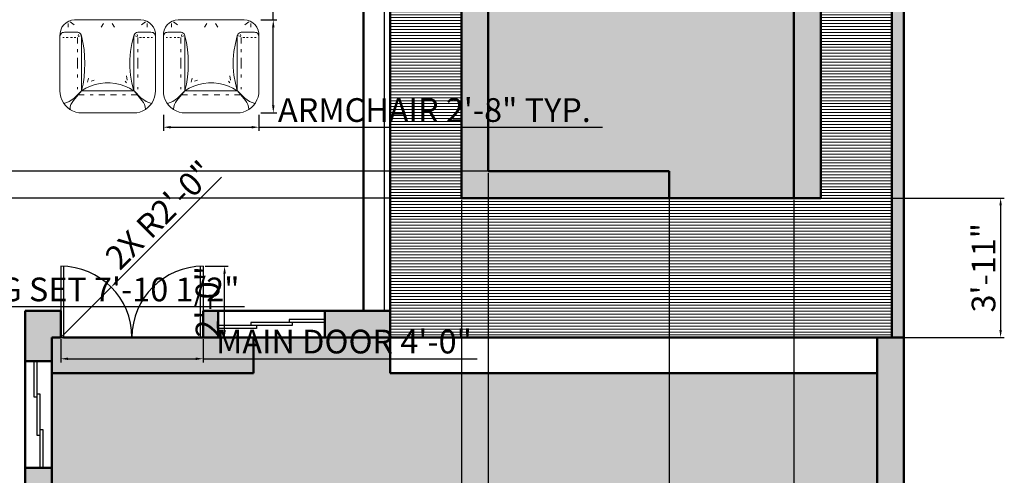
# Model space of a CAD drawing. Units: inches. Extents: x 1770 to 3141, y 984 to 1614.
# Tile 6 of 12: x 2115 to 2447, y 1254 to 1407. Entities that reach past the tile are written whole.
import ezdxf

# ---------------------------------------------------------------- set-up
doc = ezdxf.new("R2010")
doc.units = ezdxf.units.IN
for name, color, linetype, lineweight in [('A-ANNO-DIMS', 2, 'Continuous', 18), ('A-DOOR', 4, 'Continuous', 25), ('A-FLOR-PATT', 252, 'Continuous', 13), ('A-FURN', 8, 'Continuous', 18), ('A-GLAZ', 5, 'Continuous', 25), ('A-WALL', 7, 'Continuous', 50), ('A-WALL-PATT', 8, 'Continuous', 13)]:
    doc.layers.add(name, color=color, linetype=linetype, lineweight=lineweight)
doc.styles.get("Standard").update_dxf_attribs({"font": 'arial.ttf'})
doc.dimstyles.new('ISO-25', dxfattribs={"dimtxt": 8, "dimasz": 2.5, "dimexe": 1.25, "dimexo": 0.625, "dimtad": 1, "dimdec": 1, "dimlunit": 3, "dimtxsty": 'Standard', "dimcen": 2.5, "dimclrt": 1, "dimadec": 0, "dimazin": 0, "dimtfac": 1, "dimtdec": 1, "dimtmove": 0, "dimatfit": 3, "dimfxl": 1, "dimarcsym": 0})

# ---------------------------------------------------------------- blocks, each defined once
blk = doc.blocks.new("MD D 4'")
for p, q in [((0, 24), (0, 0)), ((1, 24), (1, 0)), ((47, 24), (47, 0)), ((48, 24), (48, 0)), ((0, 0), (1, 0)), ((48, 0), (47, 0))]:
    blk.add_line(p, q)
for centre, start, end in [((0, 0), 0, 90), ((48, 0), 90, 180)]:
    blk.add_arc(centre, 24, start, end)
blk = doc.blocks.new('sofa-47')
at = {"color": 0, "linetype": 'ByBlock'}
for p, q in [((-0.1449, 0.828), (-0.1656, 0.81)), ((-0.1449, 0.828), (-0.1656, 0.81)), ((-0.1206, 0.8424), (-0.1449, 0.828)), ((-0.1206, 0.8424), (-0.1449, 0.828)), ((-0.126, 0.8208), (-0.126, 0.7884)), ((-0.0945, 0.8514), (-0.1206, 0.8424)), ((-0.0945, 0.8514), (-0.1206, 0.8424)), ((-0.072, 0.8109), (-0.108, 0.8379)), ((-0.0666, 0.855), (-0.0945, 0.8514)), ((-0.0666, 0.855), (-0.0945, 0.8514)), ((0.2376, 0.855), (-0.0666, 0.855)), ((0.2376, 0.855), (-0.0666, 0.855)), ((0.1764, 0.7884), (0.198, 0.8235)), ((0.5418, 0.855), (0.2376, 0.855)), ((0.5418, 0.855), (0.2376, 0.855)), ((0.2772, 0.8235), (0.2988, 0.7884)), ((0.5697, 0.8514), (0.5418, 0.855)), ((0.5697, 0.8514), (0.5418, 0.855)), ((0.5472, 0.8109), (0.5832, 0.8379)), ((0.5958, 0.8424), (0.5697, 0.8514)), ((0.5958, 0.8424), (0.5697, 0.8514)), ((0.6201, 0.828), (0.5958, 0.8424)), ((0.6201, 0.828), (0.5958, 0.8424)), ((0.6012, 0.8208), (0.6012, 0.7884)), ((0.6408, 0.81), (0.6201, 0.828)), ((0.6408, 0.81), (0.6201, 0.828)), ((-0.2007, 0.7344), (-0.2016, 0.7065)), ((-0.2007, 0.7344), (-0.2016, 0.7065)), ((-0.1944, 0.7614), (-0.2007, 0.7344)), ((-0.1944, 0.7614), (-0.2007, 0.7344)), ((-0.1989, 0.7164), (-0.1944, 0.7254)), ((-0.1827, 0.7875), (-0.1944, 0.7614)), ((-0.1827, 0.7875), (-0.1944, 0.7614)), ((-0.1944, 0.7254), (-0.1872, 0.7326)), ((-0.1872, 0.7326), (-0.1791, 0.738)), ((-0.1656, 0.81), (-0.1827, 0.7875)), ((-0.1656, 0.81), (-0.1827, 0.7875)), ((-0.1791, 0.738), (-0.1692, 0.7407)), ((-0.1692, 0.7407), (-0.1593, 0.7416)), ((-0.1593, 0.7416), (-0.0486, 0.7416)), ((-0.0486, 0.7416), (-0.0378, 0.7416)), ((-0.0378, 0.7416), (-0.0279, 0.7389)), ((-0.0279, 0.7389), (-0.0189, 0.7335)), ((-0.0189, 0.7335), (-0.0117, 0.7263)), ((-0.0117, 0.7263), (-0.0063, 0.7182)), ((0.4815, 0.7182), (0.4869, 0.7263)), ((0.4869, 0.7263), (0.4941, 0.7335)), ((0.4941, 0.7335), (0.5031, 0.7389)), ((0.5031, 0.7389), (0.513, 0.7416)), ((0.513, 0.7416), (0.5238, 0.7416)), ((0.5238, 0.7416), (0.6345, 0.7416)), ((0.6345, 0.7416), (0.6444, 0.7407)), ((0.6579, 0.7875), (0.6408, 0.81)), ((0.6579, 0.7875), (0.6408, 0.81)), ((0.6444, 0.7407), (0.6543, 0.738)), ((0.6543, 0.738), (0.6624, 0.7326)), ((0.6696, 0.7614), (0.6579, 0.7875)), ((0.6696, 0.7614), (0.6579, 0.7875)), ((0.6624, 0.7326), (0.6696, 0.7254)), ((0.6759, 0.7344), (0.6696, 0.7614)), ((0.6759, 0.7344), (0.6696, 0.7614)), ((0.6696, 0.7254), (0.6741, 0.7164)), ((0.6768, 0.7065), (0.6759, 0.7344)), ((0.6768, 0.7065), (0.6759, 0.7344)), ((-0.2016, 0.7065), (-0.1989, 0.7164)), ((-0.2016, 0.7065), (-0.2016, 0.2034)), ((-0.2016, 0.2034), (-0.2016, 0.7065)), ((-0.1746, 0.693), (-0.162, 0.693)), ((-0.1431, 0.693), (-0.126, 0.693)), ((-0.1035, 0.693), (-0.0864, 0.693)), ((-0.072, 0.693), (-0.054, 0.693)), ((-0.0396, 0.693), (-0.0396, 0.639)), ((-0.0351, 0.7074), (-0.0324, 0.72)), ((-0.0351, 0.7029), (-0.0126, 0.7074)), ((-0.0063, 0.7182), (-0.0027, 0.7083)), ((0.0099, 0.6462), (-0.0027, 0.7083)), ((-0.0027, 0.7083), (-0.0027, 0.6975)), ((-0.0027, 0.6975), (-0.0027, 0.2034)), ((0.0198, 0.5832), (0.0099, 0.6462)), ((0.4599, 0.6372), (0.4473, 0.5652)), ((0.4779, 0.7083), (0.4599, 0.6372)), ((0.4779, 0.7083), (0.4815, 0.7182)), ((0.4779, 0.6975), (0.4779, 0.7083)), ((0.4779, 0.2034), (0.4779, 0.6975)), ((0.5103, 0.7029), (0.4878, 0.7074)), ((0.5103, 0.7074), (0.5076, 0.72)), ((0.5148, 0.693), (0.5148, 0.639)), ((0.5472, 0.693), (0.5292, 0.693)), ((0.5787, 0.693), (0.5616, 0.693)), ((0.6183, 0.693), (0.6012, 0.693)), ((0.6498, 0.693), (0.6372, 0.693)), ((0.6741, 0.7164), (0.6768, 0.7065)), ((0.6768, 0.2034), (0.6768, 0.7065)), ((0.6768, 0.7065), (0.6768, 0.2034)), ((-0.0396, 0.585), (-0.0396, 0.558)), ((0.0252, 0.5193), (0.0198, 0.5832)), ((0.4473, 0.5652), (0.441, 0.4923)), ((0.5148, 0.585), (0.5148, 0.558)), ((-0.0396, 0.4077), (-0.0396, 0.5067)), ((0.027, 0.4554), (0.0252, 0.5193)), ((0.0252, 0.3924), (0.027, 0.4554)), ((0.441, 0.4923), (0.441, 0.4194)), ((0.5148, 0.4077), (0.5148, 0.5067)), ((0.0198, 0.3285), (0.0252, 0.3924)), ((0.441, 0.4194), (0.4473, 0.3465)), ((-0.0396, 0.3267), (-0.0396, 0.3537)), ((0.0108, 0.2655), (0.0198, 0.3285)), ((0.0531, 0.2826), (0.0621, 0.3186)), ((0.0855, 0.2907), (0.1116, 0.3015)), ((0.1683, 0.2718), (0.1233, 0.2619)), ((0.2142, 0.2763), (0.1683, 0.2718)), ((0.261, 0.2763), (0.2142, 0.2763)), ((0.3069, 0.2718), (0.261, 0.2763)), ((0.3519, 0.2619), (0.3069, 0.2718)), ((0.4104, 0.2781), (0.3969, 0.2934)), ((0.4167, 0.3015), (0.4104, 0.3402)), ((0.4473, 0.3465), (0.4599, 0.2745)), ((0.4599, 0.2745), (0.4779, 0.2034)), ((0.5148, 0.3267), (0.5148, 0.3537)), ((-0.2016, 0.2034), (-0.1998, 0.1746)), ((-0.1998, 0.1746), (-0.2016, 0.2034)), ((-0.0765, 0.1152), (-0.0045, 0.2016)), ((-0.0045, 0.2016), (-0.0711, 0.135)), ((-0.0396, 0.2187), (-0.0396, 0.2358)), ((-0.0027, 0.2034), (0.0108, 0.2655)), ((0.0369, 0.2277), (-0.0027, 0.2034)), ((-0.0027, 0.2034), (0.2376, 0.2034)), ((0.0792, 0.2466), (0.0369, 0.2277)), ((0.1233, 0.2619), (0.0792, 0.2466)), ((0.2376, 0.2034), (0.4779, 0.2034)), ((0.396, 0.2466), (0.3519, 0.2619)), ((0.4383, 0.2277), (0.396, 0.2466)), ((0.4779, 0.2034), (0.4383, 0.2277)), ((0.4797, 0.2016), (0.5517, 0.1152)), ((0.5463, 0.135), (0.4797, 0.2016)), ((0.5148, 0.2187), (0.5148, 0.2358)), ((0.675, 0.1746), (0.6768, 0.2034)), ((0.6768, 0.2034), (0.675, 0.1746)), ((-0.1998, 0.1746), (-0.1935, 0.1458)), ((-0.1935, 0.1458), (-0.1998, 0.1746)), ((-0.1935, 0.1458), (-0.1836, 0.1188)), ((-0.1836, 0.1188), (-0.1935, 0.1458)), ((-0.1836, 0.1188), (-0.1701, 0.0936)), ((-0.1701, 0.0936), (-0.1836, 0.1188)), ((-0.1701, 0.0936), (-0.153, 0.0702)), ((-0.153, 0.0702), (-0.1701, 0.0936)), ((-0.1395, 0.0954), (-0.1647, 0.0873)), ((-0.1152, 0.1062), (-0.1395, 0.0954)), ((-0.0927, 0.1197), (-0.1152, 0.1062)), ((-0.0999, 0.0774), (-0.09, 0.0972)), ((-0.0711, 0.135), (-0.0927, 0.1197)), ((-0.09, 0.0972), (-0.0765, 0.1152)), ((-0.0324, 0.1647), (0.0216, 0.1647)), ((0.0756, 0.1647), (0.1026, 0.1647)), ((0.1566, 0.1647), (0.2106, 0.1647)), ((0.3186, 0.1647), (0.2646, 0.1647)), ((0.3996, 0.1647), (0.3726, 0.1647)), ((0.5076, 0.1647), (0.4536, 0.1647)), ((0.5679, 0.1197), (0.5463, 0.135)), ((0.5517, 0.1152), (0.5652, 0.0972)), ((0.5652, 0.0972), (0.5751, 0.0774)), ((0.5904, 0.1062), (0.5679, 0.1197)), ((0.6147, 0.0954), (0.5904, 0.1062)), ((0.6399, 0.0873), (0.6147, 0.0954)), ((0.6282, 0.0702), (0.6453, 0.0936)), ((0.6453, 0.0936), (0.6282, 0.0702)), ((0.6453, 0.0936), (0.6588, 0.1188)), ((0.6588, 0.1188), (0.6453, 0.0936)), ((0.6588, 0.1188), (0.6687, 0.1458)), ((0.6687, 0.1458), (0.6588, 0.1188)), ((0.6687, 0.1458), (0.675, 0.1746)), ((0.675, 0.1746), (0.6687, 0.1458)), ((-0.153, 0.0702), (-0.1323, 0.0495)), ((-0.1323, 0.0495), (-0.153, 0.0702)), ((-0.1323, 0.0495), (-0.1082, 0.0312)), ((-0.1098, 0.0324), (-0.1323, 0.0495)), ((-0.0846, 0.018), (-0.1098, 0.0324)), ((-0.1082, 0.0312), (-0.1081, 0.0315)), ((-0.1081, 0.0315), (-0.0846, 0.018)), ((-0.108, 0.0333), (-0.1062, 0.0558)), ((-0.1062, 0.0558), (-0.0999, 0.0774)), ((-0.0846, 0.018), (-0.0567, 0.0081)), ((-0.0567, 0.0081), (-0.0846, 0.018)), ((-0.0567, 0.0081), (-0.0288, 0.0018)), ((-0.0288, 0.0018), (-0.0567, 0.0081)), ((-0.0288, 0.0018), (0, 0)), ((0, 0), (-0.0288, 0.0018)), ((0, 0), (0.2376, 0)), ((0.2376, 0), (0, 0)), ((0.2376, 0), (0.4752, 0)), ((0.4752, 0), (0.2376, 0)), ((0.4752, 0), (0.504, 0.0018)), ((0.504, 0.0018), (0.4752, 0)), ((0.504, 0.0018), (0.5319, 0.0081)), ((0.5319, 0.0081), (0.504, 0.0018)), ((0.5319, 0.0081), (0.5598, 0.018)), ((0.5598, 0.018), (0.5319, 0.0081)), ((0.5598, 0.018), (0.585, 0.0324)), ((0.585, 0.0324), (0.5598, 0.018)), ((0.5751, 0.0774), (0.5814, 0.0558)), ((0.5814, 0.0558), (0.5832, 0.0333)), ((0.585, 0.0324), (0.6075, 0.0495)), ((0.6075, 0.0495), (0.585, 0.0324)), ((0.6075, 0.0495), (0.6282, 0.0702)), ((0.6282, 0.0702), (0.6075, 0.0495))]:
    blk.add_line(p, q, dxfattribs=at)
blk = doc.blocks.new('*D74')
at = {"layer": 'A-ANNO-DIMS', "color": 0, "lineweight": -2, "transparency": 16777216}
for p, q in [((2128.73, 1299.55), (2128.73, 1291.73)), ((2176.73, 1299.55), (2176.73, 1291.73)), ((2131.23, 1292.98), (2174.23, 1292.98)), ((2176.73, 1292.98), (2269.06, 1292.98))]:
    blk.add_line(p, q, dxfattribs=at)
at = {"layer": 'A-ANNO-DIMS', "color": 0, "transparency": 16777216}
for points in [[(2131.23, 1293.4), (2131.23, 1292.56), (2128.73, 1292.98)], [(2174.23, 1293.4), (2174.23, 1292.56), (2176.73, 1292.98)]]:
    blk.add_solid(points, dxfattribs=at)
at = {"layer": 'Defpoints', "color": 0, "transparency": 16777216}
for p in [(2128.73, 1300.18), (2176.73, 1300.18), (2176.73, 1292.98)]:
    blk.add_point(p, dxfattribs=at)
at = {"layer": 'A-ANNO-DIMS', "color": 1, "transparency": 16777216, "insert": (2224.15, 1297.74), "char_height": 8, "attachment_point": 5}
blk.add_mtext('MAIN DOOR 4\'-0"', dxfattribs=at)
blk = doc.blocks.new('*D75')
at = {"layer": 'A-ANNO-DIMS', "color": 0, "lineweight": -2, "transparency": 16777216}
for p, q in [((2177.36, 1324.18), (2185.18, 1324.18)), ((2183.93, 1302.68), (2183.93, 1321.68)), ((2177.36, 1300.18), (2185.18, 1300.18))]:
    blk.add_line(p, q, dxfattribs=at)
at = {"layer": 'A-ANNO-DIMS', "color": 0, "transparency": 16777216}
for points in [[(2183.52, 1321.68), (2184.35, 1321.68), (2183.93, 1324.18)], [(2183.52, 1302.68), (2184.35, 1302.68), (2183.93, 1300.18)]]:
    blk.add_solid(points, dxfattribs=at)
at = {"layer": 'Defpoints', "color": 0, "transparency": 16777216}
for p in [(2176.73, 1324.18), (2183.93, 1324.18), (2176.73, 1300.18)]:
    blk.add_point(p, dxfattribs=at)
at = {"layer": 'A-ANNO-DIMS', "color": 1, "transparency": 16777216, "insert": (2179.22, 1312.18), "char_height": 8, "attachment_point": 5, "rotation": 90}
blk.add_mtext('2\'-0"', dxfattribs=at)
blk = doc.blocks.new('*D76')
at = {"layer": 'A-ANNO-DIMS', "color": 0, "lineweight": -2, "transparency": 16777216}
for p, q in [((2163.31, 1375.26), (2163.31, 1369.8)), ((2195.51, 1375.26), (2195.51, 1369.8)), ((2165.81, 1371.05), (2193.01, 1371.05)), ((2195.51, 1371.05), (2311.2, 1371.05))]:
    blk.add_line(p, q, dxfattribs=at)
at = {"layer": 'A-ANNO-DIMS', "color": 0, "transparency": 16777216}
for points in [[(2165.81, 1371.47), (2165.81, 1370.63), (2163.31, 1371.05)], [(2193.01, 1371.47), (2193.01, 1370.63), (2195.51, 1371.05)]]:
    blk.add_solid(points, dxfattribs=at)
at = {"layer": 'Defpoints', "color": 0, "transparency": 16777216}
for p in [(2163.31, 1375.88), (2195.51, 1375.88), (2195.51, 1371.05)]:
    blk.add_point(p, dxfattribs=at)
at = {"layer": 'A-ANNO-DIMS', "color": 1, "transparency": 16777216, "insert": (2254.61, 1375.81), "char_height": 8, "attachment_point": 5}
blk.add_mtext('ARMCHAIR 2\'-8" TYP.', dxfattribs=at)
blk = doc.blocks.new('*D77')
at = {"layer": 'A-ANNO-DIMS', "color": 0, "lineweight": -2, "transparency": 16777216}
for p, q in [((2200.34, 1407.23), (2200.34, 1478.52)), ((2196.14, 1407.23), (2201.59, 1407.23)), ((2200.34, 1378.38), (2200.34, 1404.73)), ((2196.14, 1375.88), (2201.59, 1375.88))]:
    blk.add_line(p, q, dxfattribs=at)
at = {"layer": 'A-ANNO-DIMS', "color": 0, "transparency": 16777216}
for points in [[(2199.93, 1404.73), (2200.76, 1404.73), (2200.34, 1407.23)], [(2199.93, 1378.38), (2200.76, 1378.38), (2200.34, 1375.88)]]:
    blk.add_solid(points, dxfattribs=at)
at = {"layer": 'Defpoints', "color": 0, "transparency": 16777216}
for p in [(2195.51, 1407.23), (2200.34, 1407.23), (2195.51, 1375.88)]:
    blk.add_point(p, dxfattribs=at)
at = {"layer": 'A-ANNO-DIMS', "color": 1, "transparency": 16777216, "insert": (2195.58, 1444.13), "char_height": 8, "attachment_point": 5, "rotation": 90}
blk.add_mtext('2\'-7 1/2" TYP.', dxfattribs=at)
blk = doc.blocks.new('*D92')
at = {"layer": 'A-ANNO-DIMS', "color": 0, "lineweight": -2, "transparency": 16777216}
for p, q in [((1979.79, 1324.09), (1979.79, 1309.31)), ((2074.16, 1324.09), (2074.16, 1309.31)), ((1982.29, 1310.56), (2071.66, 1310.56)), ((2074.16, 1310.56), (2190.7, 1310.56))]:
    blk.add_line(p, q, dxfattribs=at)
at = {"layer": 'A-ANNO-DIMS', "color": 0, "transparency": 16777216}
for points in [[(1982.29, 1310.98), (1982.29, 1310.15), (1979.79, 1310.56)], [(2071.66, 1310.98), (2071.66, 1310.15), (2074.16, 1310.56)]]:
    blk.add_solid(points, dxfattribs=at)
at = {"layer": 'Defpoints', "color": 0, "transparency": 16777216}
for p in [(1979.79, 1324.72), (2074.16, 1324.72), (2074.16, 1310.56)]:
    blk.add_point(p, dxfattribs=at)
at = {"layer": 'A-ANNO-DIMS', "color": 1, "transparency": 16777216, "insert": (2133.68, 1315.32), "char_height": 8, "attachment_point": 5}
blk.add_mtext('DINING SET 7\'-10 1/2"', dxfattribs=at)
blk = doc.blocks.new('*D118')
at = {"layer": 'A-ANNO-DIMS', "color": 0, "lineweight": -2, "transparency": 16777216}
for p, q in [((2272.73, 1355.55), (2272.73, 991.02)), ((2263.73, 1346.55), (2263.73, 991.02)), ((2266.23, 992.27), (2270.23, 992.27)), ((2272.73, 992.27), (2297.75, 992.27))]:
    blk.add_line(p, q, dxfattribs=at)
at = {"layer": 'A-ANNO-DIMS', "color": 0, "transparency": 16777216}
for points in [[(2266.23, 992.69), (2266.23, 991.85), (2263.73, 992.27)], [(2270.23, 992.69), (2270.23, 991.85), (2272.73, 992.27)]]:
    blk.add_solid(points, dxfattribs=at)
at = {"layer": 'Defpoints', "color": 0, "transparency": 16777216}
for p in [(2272.73, 1356.18), (2263.73, 1347.18), (2272.73, 992.27)]:
    blk.add_point(p, dxfattribs=at)
at = {"layer": 'A-ANNO-DIMS', "color": 1, "transparency": 16777216, "insert": (2286.49, 996.98), "char_height": 8, "attachment_point": 5}
blk.add_mtext('0\'-9"', dxfattribs=at)
blk = doc.blocks.new('*D119')
at = {"layer": 'A-ANNO-DIMS', "color": 0, "lineweight": -2, "transparency": 16777216}
for p, q in [((2333.73, 1355.55), (2333.73, 991.02)), ((2375.73, 1346.55), (2375.73, 991.02)), ((2336.23, 992.27), (2373.23, 992.27))]:
    blk.add_line(p, q, dxfattribs=at)
at = {"layer": 'A-ANNO-DIMS', "color": 0, "transparency": 16777216}
for points in [[(2336.23, 992.69), (2336.23, 991.85), (2333.73, 992.27)], [(2373.23, 992.69), (2373.23, 991.85), (2375.73, 992.27)]]:
    blk.add_solid(points, dxfattribs=at)
at = {"layer": 'Defpoints', "color": 0, "transparency": 16777216}
for p in [(2333.73, 1356.18), (2375.73, 1347.18), (2375.73, 992.27)]:
    blk.add_point(p, dxfattribs=at)
at = {"layer": 'A-ANNO-DIMS', "color": 1, "transparency": 16777216, "insert": (2354.73, 996.98), "char_height": 8, "attachment_point": 5}
blk.add_mtext('3\'-6"', dxfattribs=at)
blk = doc.blocks.new('*D120')
at = {"layer": 'A-ANNO-DIMS', "color": 0, "lineweight": -2, "transparency": 16777216}
for p, q in [((2333.11, 1356.18), (1778.88, 1356.18)), ((1780.13, 1353.68), (1780.13, 1349.68)), ((2333.11, 1347.18), (1778.88, 1347.18)), ((1780.13, 1347.18), (1780.13, 1322.16))]:
    blk.add_line(p, q, dxfattribs=at)
at = {"layer": 'A-ANNO-DIMS', "color": 0, "transparency": 16777216}
for points in [[(1779.72, 1353.68), (1780.55, 1353.68), (1780.13, 1356.18)], [(1779.72, 1349.68), (1780.55, 1349.68), (1780.13, 1347.18)]]:
    blk.add_solid(points, dxfattribs=at)
at = {"layer": 'Defpoints', "color": 0, "transparency": 16777216}
for p in [(2333.73, 1356.18), (1780.13, 1347.18), (2333.73, 1347.18)]:
    blk.add_point(p, dxfattribs=at)
at = {"layer": 'A-ANNO-DIMS', "color": 1, "transparency": 16777216, "insert": (1775.42, 1333.42), "char_height": 8, "attachment_point": 5, "rotation": 90}
blk.add_mtext('0\'-9"', dxfattribs=at)
blk = doc.blocks.new('*D121')
at = {"layer": 'A-ANNO-DIMS', "color": 0, "lineweight": -2, "transparency": 16777216}
for p, q in [((2385.36, 1347.18), (2446.58, 1347.18)), ((2445.33, 1344.68), (2445.33, 1302.68)), ((2409.36, 1300.18), (2446.58, 1300.18))]:
    blk.add_line(p, q, dxfattribs=at)
at = {"layer": 'A-ANNO-DIMS', "color": 0, "transparency": 16777216}
for points in [[(2444.92, 1344.68), (2445.75, 1344.68), (2445.33, 1347.18)], [(2444.92, 1302.68), (2445.75, 1302.68), (2445.33, 1300.18)]]:
    blk.add_solid(points, dxfattribs=at)
at = {"layer": 'Defpoints', "color": 0, "transparency": 16777216}
for p in [(2384.73, 1347.18), (2408.73, 1300.18), (2445.33, 1300.18)]:
    blk.add_point(p, dxfattribs=at)
at = {"layer": 'A-ANNO-DIMS', "color": 1, "transparency": 16777216, "insert": (2440.62, 1323.68), "char_height": 8, "attachment_point": 5, "rotation": 90}
blk.add_mtext('3\'-11"', dxfattribs=at)
blk = doc.blocks.new('*D140')
at = {"layer": 'A-ANNO-DIMS', "color": 0, "lineweight": -2, "transparency": 16777216}
for p, q in [((2182.9, 1354.2), (2147.5, 1318.89)), ((2128.73, 1300.18), (2145.73, 1317.13))]:
    blk.add_line(p, q, dxfattribs=at)
at = {"layer": 'A-ANNO-DIMS', "color": 0, "transparency": 16777216}
blk.add_solid([(2147.2, 1319.19), (2147.79, 1318.6), (2145.73, 1317.13)], dxfattribs=at)
at = {"layer": 'Defpoints', "color": 0, "transparency": 16777216}
for p in [(2145.73, 1317.13), (2128.73, 1300.18)]:
    blk.add_point(p, dxfattribs=at)
at = {"layer": 'A-ANNO-DIMS', "color": 1, "transparency": 16777216, "insert": (2162.76, 1340.76), "char_height": 8, "attachment_point": 5, "rotation": 44.9223}
blk.add_mtext('2X R2\'-0"', dxfattribs=at)

msp = doc.modelspace()

# ---------------------------------------------------------------- hatches: boundary and pattern name
at = {"layer": 'A-FLOR-PATT'}
h = msp.add_hatch(color=256, dxfattribs=at)
h.dxf.hatch_style = 1
h.paths.add_polyline_path([(2263.73, 1565.18), (2239.73, 1565.18), (2239.73, 1561.18), (2263.73, 1561.18)])
h.paths.add_polyline_path([(2412.73, 1565.18), (2384.73, 1565.18), (2384.73, 1561.18), (2408.73, 1561.18), (2408.73, 1300.18), (2412.73, 1300.18)])
h = msp.add_hatch(color=256, dxfattribs=at)
h.dxf.hatch_style = 1
h.paths.add_polyline_path([(2384.73, 1565.18), (2263.73, 1565.18), (2263.73, 1347.18), (2333.73, 1347.18), (2333.73, 1356.18), (2272.73, 1356.18), (2272.73, 1556.18), (2375.73, 1556.18), (2375.73, 1347.18), (2384.73, 1347.18)])
h = msp.add_hatch(dxfattribs=at)
h.set_pattern_fill('_USER', color=256, pattern_type=0)
h.set_pattern_definition([(0, (0, 0), (0, 1), [])])
h.paths.add_polyline_path([(2408.73, 1561.18), (2384.73, 1561.18), (2384.73, 1347.18), (2375.73, 1347.18), (2263.73, 1347.18), (2263.73, 1561.18), (2239.73, 1561.18), (2239.73, 1300.18), (2408.73, 1300.18)])
h = msp.add_hatch(color=256, dxfattribs=at)
h.dxf.hatch_style = 1
h.paths.add_polyline_path([(2272.73, 1356.18), (2333.73, 1356.18), (2333.73, 1347.18), (2375.73, 1347.18), (2375.73, 1556.18), (2272.73, 1556.18)])
h.paths.add_polyline_path([(2287.05, 1445.97), (2372.59, 1445.97), (2372.59, 1481.19), (2287.05, 1481.19)], flags=24)
h = msp.add_hatch(color=256, dxfattribs=at)
h.dxf.hatch_style = 1
h.paths.add_polyline_path([(2403.73, 1288.18), (2239.73, 1288.18), (2239.73, 1300.18), (2193.73, 1300.18), (2193.73, 1288.18), (2125.73, 1288.18), (2125.73, 1154.18), (2125.73, 1087.18), (2280.7, 1087.18), (2280.7, 1100.18), (2289.7, 1100.18), (2289.7, 1087.18), (2403.73, 1087.18), (2403.73, 1100.18)])
h.paths.add_polyline_path([(2235.45, 1177.86), (2301.2, 1177.86), (2301.2, 1213.08), (2235.45, 1213.08)], flags=24)
h.paths.add_polyline_path([(2328.34, 1088.62), (2351.8, 1088.62), (2351.8, 1098.92), (2328.34, 1098.92)], flags=24)
h.paths.add_polyline_path([(2187.53, 1088.62), (2228.45, 1088.62), (2228.45, 1098.92), (2187.53, 1098.92)], flags=24)
at = {"layer": 'A-WALL-PATT'}
h = msp.add_hatch(color=256, dxfattribs=at)
h.dxf.hatch_style = 1
h.paths.add_polyline_path([(1821.73, 1556.18), (1844.25, 1556.18), (2086.73, 1556.18), (2086.73, 1443.18), (2091.73, 1443.18), (2091.73, 1556.18), (2239.73, 1556.18), (2239.73, 1565.18), (1812.73, 1565.18), (1812.73, 1100.18), (1821.73, 1100.18), (1821.73, 1246.18), (1913.73, 1246.18), (1913.73, 1251.18), (1821.73, 1251.18), (1821.73, 1407.18), (1944.73, 1407.18), (1944.73, 1412.18), (1821.73, 1412.18)])
h.paths.add_polyline_path([(1985.73, 1515.18), (1997.73, 1515.18), (1997.73, 1520.18), (1980.73, 1520.18), (1980.73, 1478.18), (1985.73, 1478.18)], flags=16)
h.paths.add_polyline_path([(2038.73, 1520.18), (2021.73, 1520.18), (2021.73, 1515.18), (2033.73, 1515.18), (2033.73, 1412.18), (1985.73, 1412.18), (1985.73, 1448.18), (1980.73, 1448.18), (1980.73, 1407.18), (2038.73, 1407.18), (2038.73, 1443.18), (2056.73, 1443.18), (2056.73, 1448.18), (2038.73, 1448.18)], flags=17)
h.paths.add_polyline_path([(1853.23, 1094.18), (1821.73, 1094.18), (1821.73, 1085.18), (1853.23, 1085.18)])
h.paths.add_polyline_path([(2001.73, 1094.18), (1966.73, 1094.18), (1966.73, 1124.18), (1961.73, 1124.18), (1961.73, 1094.18), (1889.23, 1094.18), (1889.23, 1085.18), (2001.73, 1085.18)])
h.paths.add_polyline_path([(2020.69, 1094.18), (2010.73, 1094.18), (2010.73, 1085.18), (2020.69, 1085.18)])
h.paths.add_polyline_path([(2116.73, 1094.18), (2080.69, 1094.18), (2080.69, 1085.18), (2116.73, 1085.18)])
h.paths.add_polyline_path([(2125.73, 1184.68), (2116.73, 1184.68), (2116.73, 1159.18), (2056.73, 1159.18), (2056.73, 1246.18), (2086.73, 1246.18), (2086.73, 1251.18), (2001.73, 1251.18), (2001.73, 1246.18), (2051.73, 1246.18), (2051.73, 1159.18), (1966.73, 1159.18), (1966.73, 1246.18), (1971.73, 1246.18), (1971.73, 1251.18), (1961.73, 1251.18), (1961.73, 1154.18), (1991.73, 1154.18), (2125.73, 1154.18)], flags=17)
h.paths.add_polyline_path([(2125.73, 1256.18), (2116.73, 1256.18), (2116.73, 1220.68), (2125.73, 1220.68)], flags=17)
h.paths.add_polyline_path([(2128.73, 1309.18), (2116.73, 1309.18), (2116.73, 1292.18), (2125.73, 1292.18), (2125.73, 1300.18), (2128.73, 1300.18)], flags=17)
h.paths.add_polyline_path([(2239.73, 1309.18), (2217.73, 1309.18), (2217.73, 1300.18), (2239.73, 1300.18)], flags=17)
h.paths.add_polyline_path([(2181.73, 1309.18), (2176.73, 1309.18), (2176.73, 1300.18), (2181.73, 1300.18)], flags=17)
h = msp.add_hatch(color=256, dxfattribs=at)
h.dxf.hatch_style = 1
h.paths.add_polyline_path([(2193.73, 1300.18), (2129.73, 1300.18), (2128.73, 1300.18), (2125.73, 1300.18), (2125.73, 1288.18), (2193.73, 1288.18)])
h = msp.add_hatch(color=256, dxfattribs=at)
h.dxf.hatch_style = 1
h.paths.add_polyline_path([(2412.73, 1300.18), (2403.73, 1300.18), (2403.73, 1100.18), (2412.73, 1100.18)])

# ---------------------------------------------------------------- linework, layer by layer
at = {"layer": 'A-GLAZ'}
for p, q in [((2237.73, 1556.18), (2237.73, 1309.18)), ((2206.73, 1304.18), (2181.73, 1304.18)), ((2217.73, 1305.18), (2192.73, 1305.18)), ((2192.73, 1305.18), (2192.73, 1304.18)), ((2194.73, 1304.18), (2194.73, 1303.18)), ((2205.73, 1306.18), (2205.73, 1305.18)), ((2217.73, 1306.18), (2205.73, 1306.18)), ((2206.73, 1305.18), (2206.73, 1304.18)), ((2194.73, 1303.18), (2181.73, 1303.18)), ((2119.73, 1292.18), (2119.73, 1280.18)), ((2120.73, 1292.18), (2120.73, 1267.18)), ((2120.73, 1281.18), (2121.73, 1281.18)), ((2121.73, 1281.18), (2121.73, 1256.18)), ((2119.73, 1280.18), (2120.73, 1280.18)), ((2120.73, 1267.18), (2121.73, 1267.18)), ((2121.73, 1269.18), (2122.73, 1269.18)), ((2122.73, 1269.18), (2122.73, 1256.18))]:
    msp.add_line(p, q, dxfattribs=at)
at = {"layer": 'A-WALL'}
for p, q in [((2239.73, 1565.18), (2239.73, 1288.18)), ((2263.73, 1565.18), (2263.73, 1347.18)), ((2384.73, 1565.18), (2384.73, 1347.18)), ((2412.73, 1565.18), (2412.73, 1043.18)), ((2408.73, 1561.18), (2408.73, 1300.18)), ((2230.73, 1556.18), (2230.73, 1309.18)), ((2272.73, 1556.18), (2272.73, 1356.18)), ((2375.73, 1556.18), (2375.73, 1347.18)), ((2272.73, 1356.18), (2333.73, 1356.18)), ((2333.73, 1356.18), (2333.73, 1347.18)), ((2263.73, 1347.18), (2375.73, 1347.18)), ((2375.73, 1347.18), (2384.73, 1347.18)), ((2116.73, 1309.18), (2128.73, 1309.18)), ((2116.73, 1159.18), (2116.73, 1309.18)), ((2128.73, 1309.18), (2128.73, 1300.18)), ((2176.73, 1309.18), (2176.73, 1300.18)), ((2176.73, 1309.18), (2239.73, 1309.18)), ((2181.73, 1309.18), (2181.73, 1300.18)), ((2217.73, 1309.18), (2217.73, 1300.18)), ((2125.73, 1300.18), (2128.73, 1300.18)), ((2125.73, 1154.18), (2125.73, 1300.18)), ((2129.73, 1300.18), (2412.73, 1300.18)), ((2193.73, 1300.18), (2193.73, 1288.18)), ((2403.73, 1300.18), (2403.73, 1085.18)), ((2116.73, 1292.18), (2125.73, 1292.18)), ((2125.73, 1288.18), (2193.73, 1288.18)), ((2239.73, 1288.18), (2403.73, 1288.18)), ((2116.73, 1256.18), (2125.73, 1256.18))]:
    msp.add_line(p, q, dxfattribs=at)

# ---------------------------------------------------------------- block references
at = {"layer": 'A-DOOR'}
msp.add_blockref("MD D 4'", (2128.73, 1300.18), dxfattribs=at)
at = {"layer": 'A-FURN', "xscale": 36.66436083614781, "yscale": 36.66436083614781, "zscale": 36.66436083614781}
for p in [(2135.86, 1375.88), (2170.7, 1375.88)]:
    msp.add_blockref('sofa-47', p, dxfattribs=at)

# ---------------------------------------------------------------- dimensions: what is measured, and where the dimension line sits
at = {"layer": 'A-ANNO-DIMS'}
dim = msp.add_linear_dim(base=(2200.3448, 1407.2305), p1=(2195.5139, 1375.8824), p2=(2195.5139, 1407.2305), angle=90, text='<> TYP.', dimstyle='ISO-25', override={"dimdec": 1, "dimrnd": 0, "dimzin": 1, "dimlunit": 4, "dimfrac": 2}, dxfattribs=at)
dim.commit()
dim.dimension.update_dxf_attribs({"geometry": '*D77', "text_midpoint": (2195.5834, 1444.1263)})
for base, p1, p2, text, picture, middle in [((2195.51, 1371.05), (2163.31, 1375.88), (2195.51, 1375.88), 'ARMCHAIR <> TYP.', '*D76', (2254.61, 1375.81)), ((2074.16, 1310.56), (1979.79, 1324.72), (2074.16, 1324.72), 'DINING SET <>', '*D92', (2133.68, 1315.32)), ((2176.73, 1292.98), (2128.73, 1300.18), (2176.73, 1300.18), 'MAIN DOOR <>', '*D74', (2224.15, 1297.74))]:
    dim = msp.add_linear_dim(base=base, p1=p1, p2=p2, text=text, dimstyle='ISO-25', override={"dimdec": 1, "dimrnd": 0, "dimzin": 1, "dimlunit": 4, "dimfrac": 2}, dxfattribs=at)
    dim.commit()
    dim.dimension.update_dxf_attribs({"geometry": picture, "text_midpoint": middle})
dim = msp.add_radius_dim(center=(2128.73, 1300.18), mpoint=(2145.73, 1317.13), text='2X <>', dimstyle='ISO-25', override={"dimdec": 1, "dimlfac": 1, "dimrnd": 0, "dimzin": 1, "dimdsep": 46, "dimlunit": 4, "dimfrac": 2}, dxfattribs=at)
dim.commit()
dim.dimension.update_dxf_attribs({"geometry": '*D140', "text_midpoint": (2162.76, 1340.76)})
for base, p1, p2, override, picture, middle in [((1780.13, 1347.18), (2333.73, 1356.18), (2333.73, 1347.18), {"dimdec": 1, "dimlfac": 1, "dimrnd": 0, "dimzin": 1, "dimdsep": 46, "dimlunit": 4, "dimfrac": 2}, '*D120', (1775.42, 1333.42)), ((2445.33, 1300.18), (2384.73, 1347.18), (2408.73, 1300.18), {"dimdec": 1, "dimlfac": 1, "dimrnd": 0, "dimzin": 1, "dimdsep": 46, "dimlunit": 4, "dimfrac": 2}, '*D121', (2440.62, 1323.68)), ((2183.93, 1324.18), (2176.73, 1300.18), (2176.73, 1324.18), {"dimdec": 1, "dimrnd": 0, "dimzin": 1, "dimlunit": 4, "dimfrac": 2}, '*D75', (2179.22, 1312.18))]:
    dim = msp.add_linear_dim(base=base, p1=p1, p2=p2, angle=90, dimstyle='ISO-25', override=override, dxfattribs=at)
    dim.commit()
    dim.dimension.update_dxf_attribs({"geometry": picture, "text_midpoint": middle})
for base, p1, p2, picture, middle in [((2272.73, 992.27), (2263.73, 1347.18), (2272.73, 1356.18), '*D118', (2286.49, 996.98)), ((2375.73, 992.27), (2333.73, 1356.18), (2375.73, 1347.18), '*D119', (2354.73, 996.98))]:
    dim = msp.add_linear_dim(base=base, p1=p1, p2=p2, dimstyle='ISO-25', override={"dimdec": 1, "dimlfac": 1, "dimrnd": 0, "dimzin": 1, "dimdsep": 46, "dimlunit": 4, "dimfrac": 2}, dxfattribs=at)
    dim.commit()
    dim.dimension.update_dxf_attribs({"geometry": picture, "text_midpoint": middle})

doc.saveas('drawing.dxf')
